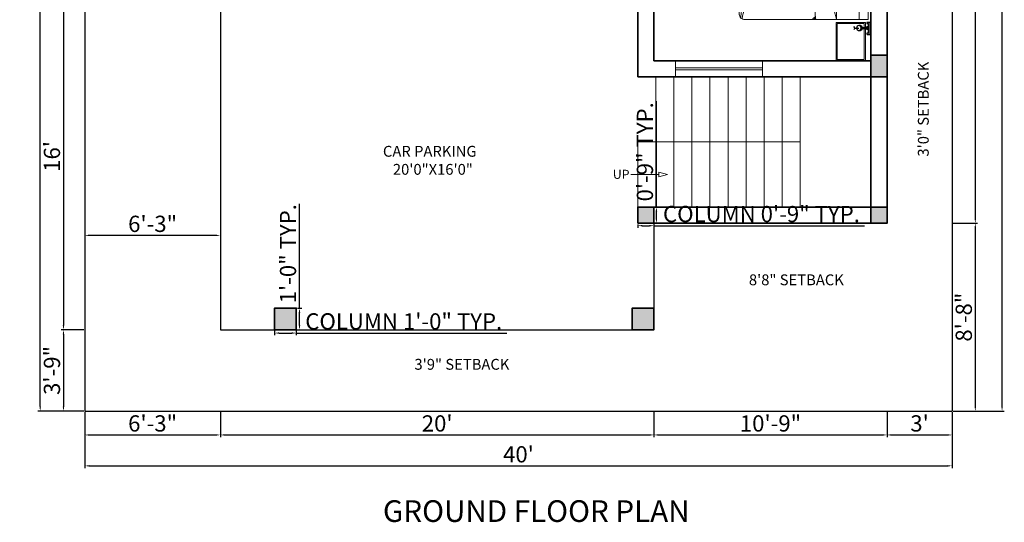
# Model space of a CAD drawing. Units: inches. Extents: x 3321 to 5237, y 11 to 1752.
# Tile 4 of 43: x 3321 to 3866, y 926 to 1204. Entities that reach past the tile are written whole.
import ezdxf

# ---------------------------------------------------------------- set-up
doc = ezdxf.new("R2010")
doc.units = ezdxf.units.IN
for name, color, linetype, lineweight in [('A-ANNO-DIMS', 2, 'Continuous', 18), ('A-ANNO-SYMB', 7, 'Continuous', 18), ('A-ANNO-TEXT', 7, 'Continuous', 18), ('A-ANNO-TITL', 7, 'Continuous', 25), ('A-AREA-IDEN', 7, 'Continuous', 18), ('A-COLS', 1, 'Continuous', 35), ('A-FLOR-EDGE', 7, 'Continuous', 25), ('A-FLOR-STRS', 7, 'Continuous', 18), ('A-GLAZ', 5, 'Continuous', 18), ('A-WALL', 7, 'Continuous', 35), ('C-PROP', 7, 'Continuous', 30), ('FUR', 42, 'Continuous', 18)]:
    doc.layers.add(name, color=color, linetype=linetype, lineweight=lineweight)
for name, color, linetype in [('CEIL', 4, 'Continuous'), ('ELEC', 4, 'Continuous'), ('wood', 26, 'Continuous')]:
    doc.layers.add(name, color=color, linetype=linetype)
doc.styles.get("Standard").update_dxf_attribs({"font": 'arial.ttf'})
doc.dimstyles.new('ISO-25', dxfattribs={"dimtxt": 9, "dimasz": 2.5, "dimexe": 1.25, "dimexo": 0.625, "dimtad": 1, "dimdec": 1, "dimlunit": 3, "dimtxsty": 'Standard', "dimcen": 2.5, "dimclrd": 4, "dimclre": 4, "dimclrt": 256, "dimadec": 0, "dimazin": 0, "dimtfac": 1, "dimtdec": 1, "dimtmove": 0, "dimatfit": 3, "dimfxl": 1, "dimarcsym": 0})

# ---------------------------------------------------------------- blocks, each defined once
blk = doc.blocks.new('*D10')
at = {"layer": 'A-ANNO-DIMS', "color": 0, "lineweight": -2, "transparency": 16777216}
for p, q in [((3356.69, 1095.75), (3356.69, 1083.38)), ((3431.69, 1095.75), (3431.69, 1083.38)), ((3429.19, 1084.63), (3359.19, 1084.63))]:
    blk.add_line(p, q, dxfattribs=at)
at = {"layer": 'A-ANNO-DIMS', "color": 0, "transparency": 16777216}
for points in [[(3359.19, 1085.05), (3359.19, 1084.21), (3356.69, 1084.63)], [(3429.19, 1085.05), (3429.19, 1084.21), (3431.69, 1084.63)]]:
    blk.add_solid(points, dxfattribs=at)
at = {"layer": 'Defpoints', "color": 0, "transparency": 16777216}
for p in [(3356.69, 1096.38), (3431.69, 1096.38), (3356.69, 1084.63)]:
    blk.add_point(p, dxfattribs=at)
at = {"layer": 'A-ANNO-DIMS', "color": 0, "transparency": 16777216, "insert": (3394.19, 1089.85), "char_height": 9, "attachment_point": 5}
blk.add_mtext('6\'-3"', dxfattribs=at)
blk = doc.blocks.new('*D32')
at = {"layer": 'A-ANNO-DIMS', "color": 0, "lineweight": -2, "transparency": 16777216}
for p, q in [((3356.06, 1224.34), (3343.59, 1224.34)), ((3344.84, 1221.84), (3344.84, 1034.84)), ((3356.06, 1032.34), (3343.59, 1032.34))]:
    blk.add_line(p, q, dxfattribs=at)
at = {"layer": 'A-ANNO-DIMS', "color": 0, "transparency": 16777216}
for points in [[(3344.42, 1221.84), (3345.26, 1221.84), (3344.84, 1224.34)], [(3344.42, 1034.84), (3345.26, 1034.84), (3344.84, 1032.34)]]:
    blk.add_solid(points, dxfattribs=at)
at = {"layer": 'Defpoints', "color": 0, "transparency": 16777216}
for p in [(3356.69, 1224.34), (3344.84, 1032.34), (3356.69, 1032.34)]:
    blk.add_point(p, dxfattribs=at)
at = {"layer": 'A-ANNO-DIMS', "color": 0, "transparency": 16777216, "insert": (3339.62, 1128.34), "char_height": 9, "attachment_point": 5, "rotation": 90}
blk.add_mtext("16'", dxfattribs=at)
blk = doc.blocks.new('*D33')
at = {"layer": 'A-ANNO-DIMS', "color": 0, "lineweight": -2, "transparency": 16777216}
for p, q in [((3356.06, 1032.34), (3343.59, 1032.34)), ((3344.84, 1029.84), (3344.84, 989.84)), ((3356.06, 987.34), (3343.59, 987.34))]:
    blk.add_line(p, q, dxfattribs=at)
at = {"layer": 'A-ANNO-DIMS', "color": 0, "transparency": 16777216}
for points in [[(3344.42, 1029.84), (3345.26, 1029.84), (3344.84, 1032.34)], [(3344.42, 989.84), (3345.26, 989.84), (3344.84, 987.34)]]:
    blk.add_solid(points, dxfattribs=at)
at = {"layer": 'Defpoints', "color": 0, "transparency": 16777216}
for p in [(3356.69, 1032.34), (3344.84, 987.34), (3356.69, 987.34)]:
    blk.add_point(p, dxfattribs=at)
at = {"layer": 'A-ANNO-DIMS', "color": 0, "transparency": 16777216, "insert": (3339.62, 1009.84), "char_height": 9, "attachment_point": 5, "rotation": 90}
blk.add_mtext('3\'-9"', dxfattribs=at)
blk = doc.blocks.new('*D34')
at = {"layer": 'A-ANNO-DIMS', "color": 0, "lineweight": -2, "transparency": 16777216}
for p, q in [((3356.69, 986.71), (3356.69, 972.86)), ((3431.69, 986.71), (3431.69, 972.86)), ((3359.19, 974.11), (3429.19, 974.11))]:
    blk.add_line(p, q, dxfattribs=at)
at = {"layer": 'A-ANNO-DIMS', "color": 0, "transparency": 16777216}
for points in [[(3359.19, 974.53), (3359.19, 973.7), (3356.69, 974.11)], [(3429.19, 974.53), (3429.19, 973.7), (3431.69, 974.11)]]:
    blk.add_solid(points, dxfattribs=at)
at = {"layer": 'Defpoints', "color": 0, "transparency": 16777216}
for p in [(3356.69, 987.34), (3431.69, 987.34), (3431.69, 974.11)]:
    blk.add_point(p, dxfattribs=at)
at = {"layer": 'A-ANNO-DIMS', "color": 0, "transparency": 16777216, "insert": (3394.19, 979.34), "char_height": 9, "attachment_point": 5}
blk.add_mtext('6\'-3"', dxfattribs=at)
blk = doc.blocks.new('*D35')
at = {"layer": 'A-ANNO-DIMS', "color": 0, "lineweight": -2, "transparency": 16777216}
for p, q in [((3431.69, 986.71), (3431.69, 972.86)), ((3671.69, 986.71), (3671.69, 972.86)), ((3434.19, 974.11), (3669.19, 974.11))]:
    blk.add_line(p, q, dxfattribs=at)
at = {"layer": 'A-ANNO-DIMS', "color": 0, "transparency": 16777216}
for points in [[(3434.19, 974.53), (3434.19, 973.7), (3431.69, 974.11)], [(3669.19, 974.53), (3669.19, 973.7), (3671.69, 974.11)]]:
    blk.add_solid(points, dxfattribs=at)
at = {"layer": 'Defpoints', "color": 0, "transparency": 16777216}
for p in [(3431.69, 987.34), (3671.69, 987.34), (3671.69, 974.11)]:
    blk.add_point(p, dxfattribs=at)
at = {"layer": 'A-ANNO-DIMS', "color": 0, "transparency": 16777216, "insert": (3551.69, 979.33), "char_height": 9, "attachment_point": 5}
blk.add_mtext("20'", dxfattribs=at)
blk = doc.blocks.new('*D36')
at = {"layer": 'A-ANNO-DIMS', "color": 0, "lineweight": -2, "transparency": 16777216}
for p, q in [((3671.69, 986.71), (3671.69, 972.86)), ((3800.69, 986.71), (3800.69, 972.86)), ((3674.19, 974.11), (3798.19, 974.11))]:
    blk.add_line(p, q, dxfattribs=at)
at = {"layer": 'A-ANNO-DIMS', "color": 0, "transparency": 16777216}
for points in [[(3674.19, 974.53), (3674.19, 973.7), (3671.69, 974.11)], [(3798.19, 974.53), (3798.19, 973.7), (3800.69, 974.11)]]:
    blk.add_solid(points, dxfattribs=at)
at = {"layer": 'Defpoints', "color": 0, "transparency": 16777216}
for p in [(3671.69, 987.34), (3800.69, 987.34), (3800.69, 974.11)]:
    blk.add_point(p, dxfattribs=at)
at = {"layer": 'A-ANNO-DIMS', "color": 0, "transparency": 16777216, "insert": (3736.19, 979.33), "char_height": 9, "attachment_point": 5}
blk.add_mtext('10\'-9"', dxfattribs=at)
blk = doc.blocks.new('*D37')
at = {"layer": 'A-ANNO-DIMS', "color": 0, "lineweight": -2, "transparency": 16777216}
for p, q in [((3800.69, 986.71), (3800.69, 972.86)), ((3836.69, 986.71), (3836.69, 972.86)), ((3803.19, 974.11), (3834.19, 974.11))]:
    blk.add_line(p, q, dxfattribs=at)
at = {"layer": 'A-ANNO-DIMS', "color": 0, "transparency": 16777216}
for points in [[(3803.19, 974.53), (3803.19, 973.7), (3800.69, 974.11)], [(3834.19, 974.53), (3834.19, 973.7), (3836.69, 974.11)]]:
    blk.add_solid(points, dxfattribs=at)
at = {"layer": 'Defpoints', "color": 0, "transparency": 16777216}
for p in [(3800.69, 987.34), (3836.69, 987.34), (3836.69, 974.11)]:
    blk.add_point(p, dxfattribs=at)
at = {"layer": 'A-ANNO-DIMS', "color": 0, "transparency": 16777216, "insert": (3818.69, 979.34), "char_height": 9, "attachment_point": 5}
blk.add_mtext("3'", dxfattribs=at)
blk = doc.blocks.new('*D42')
at = {"layer": 'A-ANNO-DIMS', "color": 0, "lineweight": -2, "transparency": 16777216}
for p, q in [((3837.31, 1635.34), (3850.8, 1635.34)), ((3849.55, 1632.84), (3849.55, 1093.84)), ((3837.31, 1091.34), (3850.8, 1091.34))]:
    blk.add_line(p, q, dxfattribs=at)
at = {"layer": 'A-ANNO-DIMS', "color": 0, "transparency": 16777216}
for points in [[(3849.13, 1632.84), (3849.96, 1632.84), (3849.55, 1635.34)], [(3849.13, 1093.84), (3849.96, 1093.84), (3849.55, 1091.34)]]:
    blk.add_solid(points, dxfattribs=at)
at = {"layer": 'Defpoints', "color": 0, "transparency": 16777216}
for p in [(3836.69, 1635.34), (3836.69, 1091.34), (3849.55, 1091.34)]:
    blk.add_point(p, dxfattribs=at)
at = {"layer": 'A-ANNO-DIMS', "color": 0, "transparency": 16777216, "insert": (3844.35, 1363.34), "char_height": 9, "attachment_point": 5, "rotation": 90}
blk.add_mtext('45\'-4"', dxfattribs=at)
blk = doc.blocks.new('*D43')
at = {"layer": 'A-ANNO-DIMS', "color": 0, "lineweight": -2, "transparency": 16777216}
for p, q in [((3837.31, 1091.34), (3850.8, 1091.34)), ((3849.55, 1088.84), (3849.55, 989.84)), ((3837.31, 987.34), (3850.8, 987.34))]:
    blk.add_line(p, q, dxfattribs=at)
at = {"layer": 'A-ANNO-DIMS', "color": 0, "transparency": 16777216}
for points in [[(3849.13, 1088.84), (3849.96, 1088.84), (3849.55, 1091.34)], [(3849.13, 989.84), (3849.96, 989.84), (3849.55, 987.34)]]:
    blk.add_solid(points, dxfattribs=at)
at = {"layer": 'Defpoints', "color": 0, "transparency": 16777216}
for p in [(3836.69, 1091.34), (3836.69, 987.34), (3849.55, 987.34)]:
    blk.add_point(p, dxfattribs=at)
at = {"layer": 'A-ANNO-DIMS', "color": 0, "transparency": 16777216, "insert": (3844.33, 1039.34), "char_height": 9, "attachment_point": 5, "rotation": 90}
blk.add_mtext('8\'-8"', dxfattribs=at)
blk = doc.blocks.new('*D45')
at = {"layer": 'A-ANNO-DIMS', "color": 0, "lineweight": -2, "transparency": 16777216}
for p, q in [((3356.06, 1707.34), (3330.71, 1707.34)), ((3331.96, 989.84), (3331.96, 1704.84)), ((3356.06, 987.34), (3330.71, 987.34))]:
    blk.add_line(p, q, dxfattribs=at)
at = {"layer": 'A-ANNO-DIMS', "color": 0, "transparency": 16777216}
for points in [[(3331.55, 1704.84), (3332.38, 1704.84), (3331.96, 1707.34)], [(3331.55, 989.84), (3332.38, 989.84), (3331.96, 987.34)]]:
    blk.add_solid(points, dxfattribs=at)
at = {"layer": 'Defpoints', "color": 0, "transparency": 16777216}
for p in [(3331.96, 1707.34), (3356.69, 1707.34), (3356.69, 987.34)]:
    blk.add_point(p, dxfattribs=at)
at = {"layer": 'A-ANNO-DIMS', "color": 0, "transparency": 16777216, "insert": (3326.74, 1347.34), "char_height": 9, "attachment_point": 5, "rotation": 90}
blk.add_mtext("60'", dxfattribs=at)
blk = doc.blocks.new('*D46')
at = {"layer": 'A-ANNO-DIMS', "color": 0, "lineweight": -2, "transparency": 16777216}
for p, q in [((3356.69, 986.71), (3356.69, 955.76)), ((3836.69, 986.71), (3836.69, 955.76)), ((3359.19, 957.01), (3834.19, 957.01))]:
    blk.add_line(p, q, dxfattribs=at)
at = {"layer": 'A-ANNO-DIMS', "color": 0, "transparency": 16777216}
for points in [[(3359.19, 957.43), (3359.19, 956.59), (3356.69, 957.01)], [(3834.19, 957.43), (3834.19, 956.59), (3836.69, 957.01)]]:
    blk.add_solid(points, dxfattribs=at)
at = {"layer": 'Defpoints', "color": 0, "transparency": 16777216}
for p in [(3356.69, 987.34), (3836.69, 987.34), (3836.69, 957.01)]:
    blk.add_point(p, dxfattribs=at)
at = {"layer": 'A-ANNO-DIMS', "color": 0, "transparency": 16777216, "insert": (3596.69, 962.23), "char_height": 9, "attachment_point": 5}
blk.add_mtext("40'", dxfattribs=at)
blk = doc.blocks.new('*D47')
at = {"layer": 'A-ANNO-DIMS', "color": 0, "lineweight": -2, "transparency": 16777216}
for p, q in [((3837.31, 1707.34), (3865.6, 1707.34)), ((3864.35, 989.84), (3864.35, 1704.84)), ((3837.31, 987.34), (3865.6, 987.34))]:
    blk.add_line(p, q, dxfattribs=at)
at = {"layer": 'A-ANNO-DIMS', "color": 0, "transparency": 16777216}
for points in [[(3863.93, 1704.84), (3864.76, 1704.84), (3864.35, 1707.34)], [(3863.93, 989.84), (3864.76, 989.84), (3864.35, 987.34)]]:
    blk.add_solid(points, dxfattribs=at)
at = {"layer": 'Defpoints', "color": 0, "transparency": 16777216}
for p in [(3836.69, 1707.34), (3864.35, 1707.34), (3836.69, 987.34)]:
    blk.add_point(p, dxfattribs=at)
at = {"layer": 'A-ANNO-DIMS', "color": 0, "transparency": 16777216, "insert": (3859.13, 1347.34), "char_height": 9, "attachment_point": 5, "rotation": 90}
blk.add_mtext("60'", dxfattribs=at)
blk = doc.blocks.new('*X127')
at = {"color": 0}
for p, q in [((3148, 8143), (3148, 8143)), ((3156, 8183), (3156, 8183)), ((3154, 7951), (3154, 7951)), ((3209, 8024), (3209, 8024)), ((3252, 7997), (3252, 7997)), ((3283, 8050), (3283, 8050))]:
    blk.add_line(p, q, dxfattribs=at)
blk = doc.blocks.new('*X126')
at = {"color": 0}
for p, q in [((3156, 8183), (3156, 8183)), ((3140, 7940), (3140, 7940))]:
    blk.add_line(p, q, dxfattribs=at)
blk = doc.blocks.new('*X125')
at = {"color": 0}
for p, q in [((3156, 8183), (3156, 8183)), ((3140, 7940), (3140, 7940))]:
    blk.add_line(p, q, dxfattribs=at)
blk = doc.blocks.new('*X124')
at = {"color": 0}
for p, q in [((3163, 7776), (3163, 7776)), ((3422, 7761), (3422, 7761)), ((3236, 7676), (3236, 7676)), ((3244, 7699), (3244, 7699)), ((3340, 7689), (3340, 7689))]:
    blk.add_line(p, q, dxfattribs=at)
blk = doc.blocks.new('BED1')
for p, q in [((0, -1000), (0, 800)), ((150, 800), (0, 800)), ((150, 800), (150, -1000)), ((2059, 800), (150, 800)), ((528, 800), (528, -1000)), ((212, 615), (277, 585)), ((2187, 355), (2187, -545)), ((2537, 405), (2237, 405)), ((2587, -545), (2587, 355)), ((2582, 188), (2565, 175)), ((2566, 179), (2565, 177)), ((2565, 175), (2586, 165)), ((2582, -287), (2565, -301)), ((2566, -297), (2565, -298)), ((2565, -301), (2586, -310)), ((2237, -595), (2537, -595)), ((150, -1000), (0, -1000)), ((150, -1000), (2063, -1000))]:
    blk.add_line(p, q)
for points in [[(934, 798), (931, 798), (928, 797), (926, 797), (925, 796), (924, 796), (923, 795), (923, 794), (922, 793), (922, 791), (922, 790), (923, 789), (923, 788), (923, 788), (922, 787), (922, 787), (921, 788), (921, 789), (920, 790), (918, 792), (917, 793), (916, 795), (915, 796), (913, 797), (912, 798), (911, 798), (910, 798), (909, 798), (908, 797), (908, 796), (907, 794), (906, 791), (905, 788), (905, 785), (904, 782), (904, 778), (903, 775), (903, 773), (903, 771), (902, 771), (902, 771), (902, 773), (902, 775), (902, 778), (902, 781), (901, 785), (901, 788), (900, 791), (899, 794), (899, 796), (898, 798), (896, 799), (895, 800), (894, 801), (893, 801), (892, 801), (891, 800), (890, 799), (889, 797), (888, 794), (888, 789), (887, 783), (886, 774), (886, 763), (885, 750), (884, 734), (884, 718), (883, 703), (882, 689), (882, 677), (882, 670), (881, 667), (881, 669), (881, 677), (881, 688), (881, 701), (881, 717), (881, 733), (880, 748), (879, 762), (878, 773), (877, 782), (875, 789), (873, 794), (870, 798), (869, 799)], [(2150, -913), (2150, 723)], [(2328, 182), (2530, 186), (2551, 182), (2562, 179), (2566, 177), (2567, 174), (2566, 172), (2562, 169), (2550, 166), (2528, 164), (2491, 162), (2345, 160), (2318, 158)], [(495, 3), (459, 95)], [(2150, -260), (2150, -268), (2150, -274), (2150, -278), (2150, -281), (2150, -284), (2150, -286), (2149, -288), (2149, -289), (2148, -290), (2147, -290), (2147, -291), (2146, -291), (2145, -291), (2144, -291), (2143, -291), (2142, -291), (2141, -291), (2141, -291), (2141, -291), (2142, -292), (2142, -293), (2144, -293), (2145, -294), (2146, -295), (2147, -297), (2148, -298), (2149, -299), (2150, -300), (2150, -300), (2150, -301), (2150, -302), (2149, -303), (2148, -303), (2147, -304), (2145, -305), (2142, -305), (2139, -306), (2136, -306), (2134, -307), (2131, -307), (2129, -307), (2128, -308), (2127, -308), (2128, -308), (2129, -308), (2131, -308), (2134, -308), (2136, -308), (2139, -309), (2142, -309), (2145, -310), (2147, -310), (2149, -311), (2150, -312), (2151, -313), (2152, -314), (2152, -315), (2152, -316), (2152, -316), (2152, -317), (2151, -318), (2149, -319), (2147, -319), (2143, -320), (2137, -321), (2130, -321), (2121, -322), (2110, -322), (2097, -323), (2084, -323), (2071, -324), (2059, -324), (2050, -325), (2043, -325), (2041, -325), (2043, -325), (2049, -325), (2058, -325), (2070, -325), (2082, -325), (2096, -326), (2108, -326), (2120, -327), (2129, -328), (2137, -329), (2143, -330), (2147, -332), (2150, -334), (2151, -336)], [(2247, -294), (2530, -289), (2551, -293), (2562, -296), (2566, -299), (2567, -301), (2566, -303), (2562, -306), (2550, -309), (2528, -311), (2491, -313), (2345, -315), (2239, -322)], [(1734, -998), (1731, -998), (1729, -998), (1727, -997), (1726, -997), (1725, -996), (1725, -996), (1724, -995), (1724, -994), (1724, -993), (1724, -992), (1724, -991), (1724, -990), (1724, -990), (1724, -989), (1724, -989), (1723, -990), (1723, -991), (1722, -992), (1721, -993), (1720, -994), (1719, -996), (1718, -997), (1717, -998), (1716, -998), (1715, -999), (1714, -999), (1713, -998), (1712, -998), (1712, -996), (1711, -995), (1710, -993), (1710, -990), (1709, -988), (1709, -985), (1708, -982), (1708, -979), (1708, -977), (1707, -976), (1707, -976), (1707, -976), (1707, -977), (1707, -979), (1707, -982), (1707, -985), (1706, -987), (1706, -990), (1706, -993), (1705, -995), (1704, -997), (1703, -998), (1702, -999), (1701, -1000), (1701, -1000), (1700, -1001), (1699, -1000), (1698, -1000), (1697, -999), (1696, -998), (1696, -995), (1695, -991), (1694, -986), (1694, -979), (1693, -969), (1693, -958), (1692, -945), (1692, -932), (1691, -919), (1691, -907), (1690, -898), (1690, -891), (1690, -889), (1690, -891), (1690, -897), (1690, -906), (1690, -918), (1690, -931), (1689, -944), (1689, -957), (1688, -968), (1687, -978), (1686, -985), (1685, -991), (1683, -995), (1681, -998), (1680, -999)]]:
    blk.add_lwpolyline(points)
for points in [[(205, 620, 0.267769), (215, 582, -0.037739), (204, 22, 0.684696), (237, 6, -0.060702), (497, 0, -0.046649), (226, 3, -1.318436)], [(489, 620, 0.144019), (208, 618, 0.248643)], [(497, 0, 0.021276), (489, 620, -0.206383), (327, 509, 0.237198)], [(212, 13, 0.143972), (362, 263, 1.292232)], [(886, -150, -0.069098), (985, -67, 0.658965), (982, -49, -0.049789), (927, -29, -0.103757), (897, -5, 0.055725), (801, 83, -0.11866), (783, 105, 0.016811), (762, 144, 0.70791), (748, 144, -0.16964), (552, -97, 0.664036), (554, -111, 0.023706), (627, -145, -0.134834), (683, -188, 0.012748), (746, -267)], [(489, -168, 0.144019), (208, -170, 0.248643)], [(969, -259, 0.263265), (936, -237, -0.026108), (909, -233, 0.027613), (945, -234, -0.089259), (873, -120, 0.662242), (858, -119, -0.162037), (652, -333, 0.676499), (654, -355, -0.160513), (723, -401, 0.07473), (774, -450, -0.187721), (846, -560, 0.70791), (859, -561, -0.010003), (899, -497, -0.113819), (947, -450, 0.099539), (1033, -372, -0.173425), (1071, -346, 0.589988), (1076, -326, 0.137312), (924, -246, 0.137312)], [(205, -168, 0.267769), (215, -205, -0.037739), (204, -766, 0.684696), (237, -782, -0.060702), (497, -788, -0.046649), (226, -785, -1.318436)], [(497, -788, 0.021276), (489, -168, -0.206383), (327, -278, 0.237198)], [(1446, -733, -0.095039), (653, -1002)]]:
    blk.add_lwpolyline(points, format="xyb")
for centre, radius, start, end in [((3209, 1363), 2739, 191.8679, 206.3247), ((1139, 794), 983, 294.6078, 358.3033), ((1608, 843), 496, 305.1901, 354.0206), ((2063, 714), 86.5, 0, 93.5376), ((2099, 755), 1625, 193.905, 207.8169), ((2237, 355), 50, 90, 180), ((2202, 323), 34.8, 50.8413, 114.9586), ((2212, 381), 36.5, 226.8095, 258.3841), ((2227, 374), 32.8, 17.833, 72.8005), ((2321, 410), 84.5, 185.6196, 217.1396), ((2547, 374), 32.8, 107.1995, 162.167), ((2453, 410), 84.5, 322.8604, 354.3804), ((2537, 355), 50, 0, 90), ((2573, 323), 34.8, 65.0414, 129.1587), ((2562, 381), 36.5, 281.6159, 313.1905), ((341, -278), 318, 60.7125, 115.009), ((752, 89), 34.9, 336.8352, 27.7218), ((684, 86), 100, 353.675, 10.882), ((1074, 199), 306, 197.8602, 241.5122), ((602, -324), 199, 43.2035, 95.0556), ((3209, 1363), 2739, 212.9314, 216.951), ((984, -79), 20.8, 73.7967, 130.4566), ((978, -69), 14.3, 39.7097, 85.9506), ((980, -379), 163, 152.6104, 209.361), ((981, -282), 131, 164.0372, 243.4536), ((2099, 755), 1625, 226.5887, 246.3156), ((3209, 1363), 2739, 218.6329, 229.9449), ((3403, -343), 1409, 182.9917, 205.6819), ((-34, -471), 377, 312.0118, 350.9635), ((2188, -476), 73, 269.4513, 322.8027), ((2178, -513), 33, 286.1827, 338.1386), ((2237, -545), 50, 180, 270), ((2271, -581), 35.8, 148.9055, 197.5541), ((2547, -564), 32.8, 197.833, 252.8005), ((2453, -600), 84.5, 5.6196, 37.1396), ((2537, -545), 50, 270, 0), ((2573, -514), 34.8, 230.8413, 294.9586), ((2562, -572), 36.5, 46.8095, 78.3841), ((341, -1065), 318, 60.7125, 115.009), ((376, -807), 128, 17.4073, 88.5129), ((1929, -1126), 250, 37.8553, 88.4405), ((2063, -913), 86.5, 270, 0)]:
    blk.add_arc(centre, radius, start, end)
for name in ['*X126', '*X125', '*X127', '*X124']:
    blk.add_blockref(name, (-2425, -8101))
blk = doc.blocks.new('APLIQ')
at = {"layer": 'ELEC'}
for p, q in [((0, 0.2), (-0.026, 0.226)), ((0, 0.2), (0.026, 0.226)), ((0, 0.2), (0, 0.14)), ((-0.05, 0.14), (-0.04, 0.14)), ((-0.03, 0.01), (0.03, 0.01)), ((-0.03, 0), (0.03, 0)), ((-0.01, 0.09), (-0.01, 0.01)), ((0, 0.09), (0, 0)), ((0.01, 0.09), (0.01, 0.01)), ((0.04, 0.14), (0.05, 0.14))]:
    blk.add_line(p, q, dxfattribs=at)
blk.add_circle((0, 0.14), 0.04, dxfattribs=at)
blk.add_arc((0, 0.14), 0.05, 180, 0, dxfattribs=at)
blk = doc.blocks.new('A$C68AE1801')
at = {"layer": 'FUR'}
for points in [[(2.542, 3.18), (2.542, 2.54), (2.052, 2.54), (2.052, 3.18)], [(2.522, 3.16), (2.522, 2.56), (2.072, 2.56), (2.072, 3.16)], [(2.542, 0), (2.542, 0.64), (2.052, 0.64), (2.052, 0)], [(2.522, 0.02), (2.522, 0.62), (2.072, 0.62), (2.072, 0.02)]]:
    blk.add_lwpolyline(points, close=True, dxfattribs=at)
at = {"layer": 'wood'}
for p, q in [((2.606, 2.74), (2.606, 2.54)), ((2.606, 0.44), (2.606, 0.64))]:
    blk.add_line(p, q, dxfattribs=at)
for points in [[(2.566, 2.728), (2.566, 2.732, -0.414214), (2.574, 2.74), (2.632, 2.74), (2.632, 2.54), (2.574, 2.54, -0.414214), (2.566, 2.548), (2.566, 2.552, -0.414214), (2.574, 2.56), (2.578, 2.56, 0.414214), (2.586, 2.568), (2.586, 2.712, 0.414214), (2.578, 2.72), (2.574, 2.72, -0.414214)], [(2.566, 0.452), (2.566, 0.448, 0.414214), (2.574, 0.44), (2.632, 0.44), (2.632, 0.64), (2.574, 0.64, 0.414214), (2.566, 0.632), (2.566, 0.628, 0.414214), (2.574, 0.62), (2.578, 0.62, -0.414214), (2.586, 0.612), (2.586, 0.468, -0.414214), (2.578, 0.46), (2.574, 0.46, 0.414214)]]:
    blk.add_lwpolyline(points, format="xyb", close=True, dxfattribs=at)
at = {"layer": 'CEIL', "rotation": 90}
blk.add_blockref('APLIQ', (2.574, 2.634), dxfattribs=at)
at = {"layer": 'CEIL', "xscale": -1, "rotation": 90}
blk.add_blockref('APLIQ', (2.574, 0.546), dxfattribs=at)
at = {"layer": 'FUR', "xscale": 0.001, "yscale": 0.001, "zscale": 0.001, "rotation": 180}
blk.add_blockref('BED1', (2.587, 1.49), dxfattribs=at)
blk = doc.blocks.new('COL-9X12-FURN-PLAN')
h = blk.add_hatch(color=256)
h.dxf.hatch_style = 1
h.paths.add_polyline_path([(0, 12), (0, 0), (9, 0), (9, 12)])
blk.add_lwpolyline([(0, 0), (9, 0), (9, 12), (0, 12)], close=True)
blk = doc.blocks.new('COL-9X9-FURN-PLAN')
h = blk.add_hatch(color=256)
h.dxf.hatch_style = 1
h.paths.add_polyline_path([(9, 9), (0, 9), (0, 0), (9, 0)])
blk.add_lwpolyline([(0, 0), (9, 0), (9, 9), (0, 9)], close=True)
blk = doc.blocks.new('COL-12X12-FURN-PLAN')
h = blk.add_hatch(color=256)
h.dxf.hatch_style = 1
h.paths.add_polyline_path([(12, 0), (12, 12), (0, 12), (0, 0)])
blk.add_lwpolyline([(0, 0), (12, 0), (12, 12), (0, 12)], close=True)
blk = doc.blocks.new('WIN-48IN-9IN-WALL')
for p, q in [((0, 0), (0, 9)), ((48, 0), (48, 9)), ((0, 5), (48, 5)), ((0, 4), (48, 4))]:
    blk.add_line(p, q)
blk = doc.blocks.new('STAIR-RETURN-72IN')
for p, q in [((10, 72), (10, 0)), ((20, 72), (20, 0)), ((30, 72), (30, 0)), ((40, 72), (40, 0)), ((50, 72), (50, 0)), ((60, 72), (60, 0)), ((70, 72), (70, 0)), ((80, 72), (80, 0)), ((90, 72), (90, 0)), ((90, 36), (0, 36)), ((0, 36), (0, 0))]:
    blk.add_line(p, q)
blk = doc.blocks.new('STAIR-DIRECTION-ARROW')
blk.add_line((0, 1.22), (15.43, 1.22))
blk.add_lwpolyline([(20.27, 1.22), (15.43, 2.43), (15.43, 0)], close=True)
blk = doc.blocks.new('PROPERTY-40X60FT')
for p, q in [((0, 720), (480, 720)), ((0, 720), (0, 0)), ((480, 720), (480, 0)), ((0, 0), (480, 0))]:
    blk.add_line(p, q)
blk = doc.blocks.new('*D179')
at = {"layer": 'A-ANNO-DIMS', "color": 4, "lineweight": -2, "transparency": 16777216}
for p, q in [((3662.69, 1090.71), (3662.69, 1088.74)), ((3665.19, 1089.99), (3669.19, 1089.99)), ((3671.69, 1090.71), (3671.69, 1088.74)), ((3671.69, 1089.99), (3788.17, 1089.99))]:
    blk.add_line(p, q, dxfattribs=at)
at = {"layer": 'A-ANNO-DIMS', "color": 4, "transparency": 16777216}
for points in [[(3665.19, 1090.41), (3665.19, 1089.57), (3662.69, 1089.99)], [(3669.19, 1090.41), (3669.19, 1089.57), (3671.69, 1089.99)]]:
    blk.add_solid(points, dxfattribs=at)
at = {"layer": 'Defpoints', "color": 0, "transparency": 16777216}
for p in [(3662.69, 1091.34), (3671.69, 1091.34), (3671.69, 1089.99)]:
    blk.add_point(p, dxfattribs=at)
at = {"layer": 'A-ANNO-DIMS', "transparency": 16777216, "insert": (3731.18, 1095.27), "char_height": 9, "attachment_point": 5}
blk.add_mtext('COLUMN 0\'-9" TYP.', dxfattribs=at)
blk = doc.blocks.new('*D180')
at = {"layer": 'A-ANNO-DIMS', "color": 4, "lineweight": -2, "transparency": 16777216}
for p, q in [((3673.04, 1100.34), (3673.04, 1158.95)), ((3672.31, 1100.34), (3674.29, 1100.34)), ((3673.04, 1093.84), (3673.04, 1097.84)), ((3672.31, 1091.34), (3674.29, 1091.34))]:
    blk.add_line(p, q, dxfattribs=at)
at = {"layer": 'A-ANNO-DIMS', "color": 4, "transparency": 16777216}
for points in [[(3672.62, 1097.84), (3673.46, 1097.84), (3673.04, 1100.34)], [(3672.62, 1093.84), (3673.46, 1093.84), (3673.04, 1091.34)]]:
    blk.add_solid(points, dxfattribs=at)
at = {"layer": 'Defpoints', "color": 0, "transparency": 16777216}
for p in [(3671.69, 1100.34), (3673.04, 1100.34), (3671.69, 1091.34)]:
    blk.add_point(p, dxfattribs=at)
at = {"layer": 'A-ANNO-DIMS', "transparency": 16777216, "insert": (3667.82, 1130.89), "char_height": 9, "attachment_point": 5, "rotation": 90}
blk.add_mtext('0\'-9" TYP.', dxfattribs=at)
blk = doc.blocks.new('*D181')
at = {"layer": 'A-ANNO-DIMS', "color": 4, "lineweight": -2, "transparency": 16777216}
for p, q in [((3461.69, 1031.71), (3461.69, 1029.29)), ((3464.19, 1030.54), (3471.19, 1030.54)), ((3473.69, 1031.71), (3473.69, 1029.29)), ((3473.69, 1030.54), (3590.17, 1030.54))]:
    blk.add_line(p, q, dxfattribs=at)
at = {"layer": 'A-ANNO-DIMS', "color": 4, "transparency": 16777216}
for points in [[(3464.19, 1030.96), (3464.19, 1030.12), (3461.69, 1030.54)], [(3471.19, 1030.96), (3471.19, 1030.12), (3473.69, 1030.54)]]:
    blk.add_solid(points, dxfattribs=at)
at = {"layer": 'Defpoints', "color": 0, "transparency": 16777216}
for p in [(3461.69, 1032.34), (3473.69, 1032.34), (3473.69, 1030.54)]:
    blk.add_point(p, dxfattribs=at)
at = {"layer": 'A-ANNO-DIMS', "transparency": 16777216, "insert": (3533.18, 1035.82), "char_height": 9, "attachment_point": 5}
blk.add_mtext('COLUMN 1\'-0" TYP.', dxfattribs=at)
blk = doc.blocks.new('*D182')
at = {"layer": 'A-ANNO-DIMS', "color": 4, "lineweight": -2, "transparency": 16777216}
for p, q in [((3475.49, 1044.34), (3475.49, 1102.1)), ((3474.31, 1044.34), (3476.74, 1044.34)), ((3475.49, 1034.84), (3475.49, 1041.84)), ((3474.31, 1032.34), (3476.74, 1032.34))]:
    blk.add_line(p, q, dxfattribs=at)
at = {"layer": 'A-ANNO-DIMS', "color": 4, "transparency": 16777216}
for points in [[(3475.07, 1041.84), (3475.91, 1041.84), (3475.49, 1044.34)], [(3475.07, 1034.84), (3475.91, 1034.84), (3475.49, 1032.34)]]:
    blk.add_solid(points, dxfattribs=at)
at = {"layer": 'Defpoints', "color": 0, "transparency": 16777216}
for p in [(3473.69, 1044.34), (3475.49, 1044.34), (3473.69, 1032.34)]:
    blk.add_point(p, dxfattribs=at)
at = {"layer": 'A-ANNO-DIMS', "transparency": 16777216, "insert": (3470.27, 1074.47), "char_height": 9, "attachment_point": 5, "rotation": 90}
blk.add_mtext('1\'-0" TYP.', dxfattribs=at)

msp = doc.modelspace()

# ---------------------------------------------------------------- linework, layer by layer
at = {"layer": 'A-FLOR-EDGE'}
for p, q in [((3431.69, 1224.34), (3431.69, 1032.34)), ((3671.69, 1091.34), (3671.69, 1032.34)), ((3431.69, 1032.34), (3671.69, 1032.34))]:
    msp.add_line(p, q, dxfattribs=at)
at = {"layer": 'A-WALL'}
for p, q in [((3800.69, 1635.34), (3800.69, 1091.34)), ((3791.69, 1316.34), (3791.69, 1181.34)), ((3671.69, 1271.34), (3671.69, 1181.34)), ((3662.69, 1224.34), (3662.69, 1172.34)), ((3671.69, 1181.34), (3791.69, 1181.34)), ((3662.69, 1172.34), (3791.69, 1172.34)), ((3791.69, 1172.34), (3791.69, 1100.34)), ((3662.69, 1100.34), (3791.69, 1100.34)), ((3662.69, 1100.34), (3662.69, 1091.34)), ((3662.69, 1091.34), (3800.69, 1091.34))]:
    msp.add_line(p, q, dxfattribs=at)

# ---------------------------------------------------------------- block references
at = {"layer": 'A-ANNO-SYMB'}
msp.add_blockref('STAIR-DIRECTION-ARROW', (3658.96, 1117.12), dxfattribs=at)
at = {"layer": 'A-COLS'}
for name, p in [('COL-9X12-FURN-PLAN', (3791.69, 1172.34)), ('COL-9X9-FURN-PLAN', (3662.69, 1091.34)), ('COL-9X9-FURN-PLAN', (3791.69, 1091.34)), ('COL-12X12-FURN-PLAN', (3461.69, 1032.34)), ('COL-12X12-FURN-PLAN', (3659.69, 1032.34))]:
    msp.add_blockref(name, p, dxfattribs=at)
at = {"layer": 'A-FLOR-STRS'}
msp.add_blockref('STAIR-RETURN-72IN', (3662.69, 1100.34), dxfattribs=at)
at = {"layer": 'A-GLAZ'}
msp.add_blockref('WIN-48IN-9IN-WALL', (3683.69, 1172.34), dxfattribs=at)
at = {"layer": 'C-PROP'}
msp.add_blockref('PROPERTY-40X60FT', (3356.69, 987.34), dxfattribs=at)
at = {"layer": 'FUR', "xscale": 33.17188472218209, "yscale": 33.17188472218209, "zscale": 33.17188472218209}
msp.add_blockref('A$C68AE1801', (3704.38, 1181.34), dxfattribs=at)

# ---------------------------------------------------------------- texts
at = {"layer": 'A-ANNO-TEXT'}
msp.add_text('UP', height=5, dxfattribs=at).set_placement((3648.91, 1115.94))
at = {"layer": 'A-ANNO-TEXT', "insert": (3817.76, 1128.26), "char_height": 6, "attachment_point": 1, "rotation": 90}
msp.add_mtext_dynamic_manual_height_columns('3\'0" SETBACK', width=97.3114, gutter_width=25, heights=[0], dxfattribs=at)
at = {"layer": 'A-ANNO-TEXT', "char_height": 6, "attachment_point": 1}
for s, insert in [('8\'8" SETBACK', (3724.23, 1063.01)), ('3\'9" SETBACK', (3539.12, 1016.23))]:
    msp.add_mtext_dynamic_manual_height_columns(s, width=97.3114, gutter_width=25, heights=[0], dxfattribs=dict(at, insert=insert))
at = {"layer": 'A-ANNO-TITL', "insert": (3521.67, 937.95), "char_height": 12, "attachment_point": 1}
msp.add_mtext_dynamic_manual_height_columns('GROUND FLOOR PLAN', width=241.3793, gutter_width=25, heights=[0], dxfattribs=at)
at = {"layer": 'A-AREA-IDEN', "insert": (3521.67, 1134.19), "char_height": 6, "attachment_point": 1}
msp.add_mtext_dynamic_manual_height_columns('CAR PARKING\\P   20\'0"X16\'0"', width=108.2268, gutter_width=25, heights=[0], dxfattribs=at)

# ---------------------------------------------------------------- dimensions: what is measured, and where the dimension line sits
at = {"layer": 'A-ANNO-DIMS'}
for base, p1, p2, angle, override, picture, middle in [((3331.96, 1707.34), (3356.69, 987.34), (3356.69, 1707.34), 270, {"dimclrd": 0, "dimclre": 0, "dimclrt": 0}, '*D45', (3326.74, 1347.34)), ((3864.35, 1707.34), (3836.69, 987.34), (3836.69, 1707.34), 270, {"dimclrd": 0, "dimclre": 0, "dimclrt": 0}, '*D47', (3859.13, 1347.34)), ((3849.55, 1091.34), (3836.69, 1635.34), (3836.69, 1091.34), 90, {"dimclrd": 0, "dimclre": 0, "dimclrt": 0, "dimtmove": 1}, '*D42', (3844.35, 1363.34)), ((3344.84, 1032.34), (3356.69, 1224.34), (3356.69, 1032.34), 90, {"dimclrd": 0, "dimclre": 0, "dimclrt": 0, "dimtmove": 1}, '*D32', (3339.62, 1128.34)), ((3849.55, 987.34), (3836.69, 1091.34), (3836.69, 987.34), 90, {"dimclrd": 0, "dimclre": 0, "dimclrt": 0, "dimtmove": 1}, '*D43', (3844.33, 1039.34)), ((3344.84, 987.34), (3356.69, 1032.34), (3356.69, 987.34), 90, {"dimclrd": 0, "dimclre": 0, "dimclrt": 0, "dimtmove": 1}, '*D33', (3339.62, 1009.84))]:
    dim = msp.add_linear_dim(base=base, p1=p1, p2=p2, angle=angle, dimstyle='ISO-25', override=override, dxfattribs=at)
    dim.commit()
    dim.dimension.update_dxf_attribs({"geometry": picture, "text_midpoint": middle})
for base, p1, p2, picture, middle in [((3673.04, 1100.34), (3671.69, 1091.34), (3671.69, 1100.34), '*D180', (3667.82, 1130.89)), ((3475.49, 1044.34), (3473.69, 1032.34), (3473.69, 1044.34), '*D182', (3470.27, 1074.47))]:
    dim = msp.add_linear_dim(base=base, p1=p1, p2=p2, angle=90, text='<> TYP.', dimstyle='ISO-25', override={"dimdec": 1, "dimlfac": 1, "dimrnd": 0, "dimzin": 1, "dimdsep": 46, "dimlunit": 4, "dimfrac": 2}, dxfattribs=at)
    dim.commit()
    dim.dimension.update_dxf_attribs({"geometry": picture, "text_midpoint": middle})
for base, p1, p2, picture, middle in [((3671.69, 1089.99), (3662.69, 1091.34), (3671.69, 1091.34), '*D179', (3731.18, 1095.27)), ((3473.69, 1030.54), (3461.69, 1032.34), (3473.69, 1032.34), '*D181', (3533.18, 1035.82))]:
    dim = msp.add_linear_dim(base=base, p1=p1, p2=p2, text='COLUMN <> TYP.', dimstyle='ISO-25', override={"dimdec": 1, "dimlfac": 1, "dimrnd": 0, "dimzin": 1, "dimdsep": 46, "dimlunit": 4, "dimfrac": 2}, dxfattribs=at)
    dim.commit()
    dim.dimension.update_dxf_attribs({"geometry": picture, "text_midpoint": middle})
for base, p1, p2, override, picture, middle in [((3356.69, 1084.63), (3431.69, 1096.38), (3356.69, 1096.38), {"dimclrd": 0, "dimclre": 0, "dimclrt": 0}, '*D10', (3394.19, 1089.85)), ((3431.69, 974.11), (3356.69, 987.34), (3431.69, 987.34), {"dimclrd": 0, "dimclre": 0, "dimclrt": 0}, '*D34', (3394.19, 979.34)), ((3836.69, 957.01), (3356.69, 987.34), (3836.69, 987.34), {"dimclrd": 0, "dimclre": 0, "dimclrt": 0}, '*D46', (3596.69, 962.23)), ((3671.69, 974.11), (3431.69, 987.34), (3671.69, 987.34), {"dimclrd": 0, "dimclre": 0, "dimclrt": 0, "dimtmove": 1}, '*D35', (3551.69, 979.33)), ((3800.69, 974.11), (3671.69, 987.34), (3800.69, 987.34), {"dimclrd": 0, "dimclre": 0, "dimclrt": 0, "dimtmove": 1}, '*D36', (3736.19, 979.33)), ((3836.69, 974.11), (3800.69, 987.34), (3836.69, 987.34), {"dimclrd": 0, "dimclre": 0, "dimclrt": 0, "dimtmove": 1}, '*D37', (3818.69, 979.34))]:
    dim = msp.add_linear_dim(base=base, p1=p1, p2=p2, dimstyle='ISO-25', override=override, dxfattribs=at)
    dim.commit()
    dim.dimension.update_dxf_attribs({"geometry": picture, "text_midpoint": middle})

doc.saveas('drawing.dxf')
